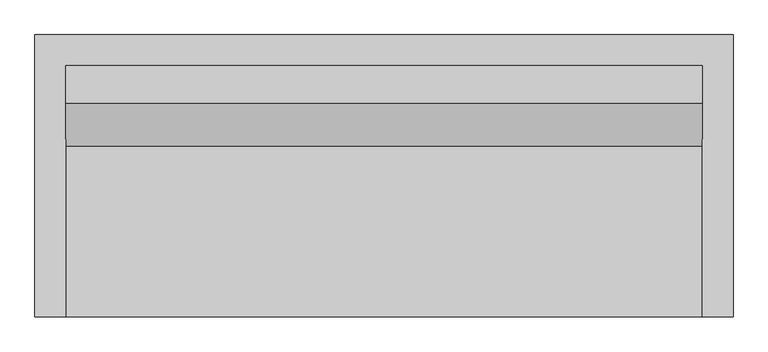
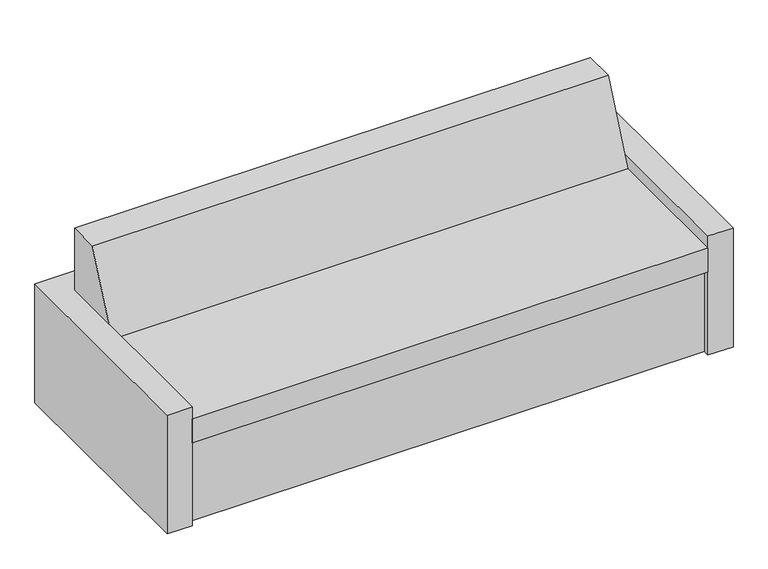
"""IFC4 building model written with IfcOpenShell, lengths in millimetres: furniture geometry."""

from ifc_helpers import new_model, si_unit, frame, origin, origin_with_axes, place, context, project, spatial, polyline, outline, extrude, source, transform, mapped, element, save


def furniture_47c73875(model_context):
    return source(origin(), model_context, "Body", "SweptSolid", [
        extrude(outline(polyline([(-359.4256442, 450.0), (-222.4208629, 760.0), (-100.0, 760.0), (-100.0, 0.0), (-884.6, 0.0), (-884.6, 348.4), (-910.0, 348.4), (-910.0, 450.0), (-359.4256442, 450.0)])), frame((-948.8, 0.0, 0.0), z_axis=(1.0, 0.0, 0.0), x_axis=(0.0, 1.0, 0.0)), (0.0, 0.0, 1.0), 2050.0),
        extrude(outline(polyline([(1201.2, 0.0), (1201.2, -910.0), (1101.2, -910.0), (1101.2, -100.0), (-948.8, -100.0), (-948.8, -910.0), (-1048.8, -910.0), (-1048.8, 0.0), (1201.2, 0.0)])), origin_with_axes(), (0.0, 0.0, 1.0), 500.0),
    ])


if __name__ == "__main__":
    model = new_model("IFC4")
    model_context = context("Model", 3, world=origin())
    ifc_project = project(units=[si_unit("LENGTHUNIT", "METRE", prefix="MILLI")], contexts=[model_context])
    site = spatial("IfcSite", under=ifc_project)
    building = spatial("IfcBuilding", under=site)
    placement = place(None, origin())
    furniture_shape = furniture_47c73875(model_context)
    element("IfcFurniture", 1, at=placement, inside=building, context=model_context, shape_type="MappedRepresentation", body=[
        mapped(furniture_shape, transform((0.0, 0.0, 0.0), x_axis=(1.0, 0.0, 0.0), y_axis=(0.0, 1.0, 0.0), z_axis=(0.0, 0.0, 1.0))),
    ])
    save(model, "model.ifc")

# Revit data of these elements
# Type
#   width = 2250 mm
#   seat height = 450 mm
#   height = 760 mm
#   depth = 910 mm
#   arm height = 500 mm
#   arm depth = 100 mm
#   Total Seat Room = 2050 mm
#   Seat Width = 683.333 mm
#   Seat Count = 3
#   Is Mark Visible = yes
#   seat material = Sofa seat
#   arm material = Sofa arm
#   Default Elevation = 0
#   Assembly Code = ""
# Element 1 (IfcFurniture)
#   Materials on its faces: "Sofa seat", "Sofa arm"
# Materials
#   "Sofa seat": colour RGB 247 247 239, transparency 0
#   "Sofa arm": colour RGB 247 247 239, transparency 0
